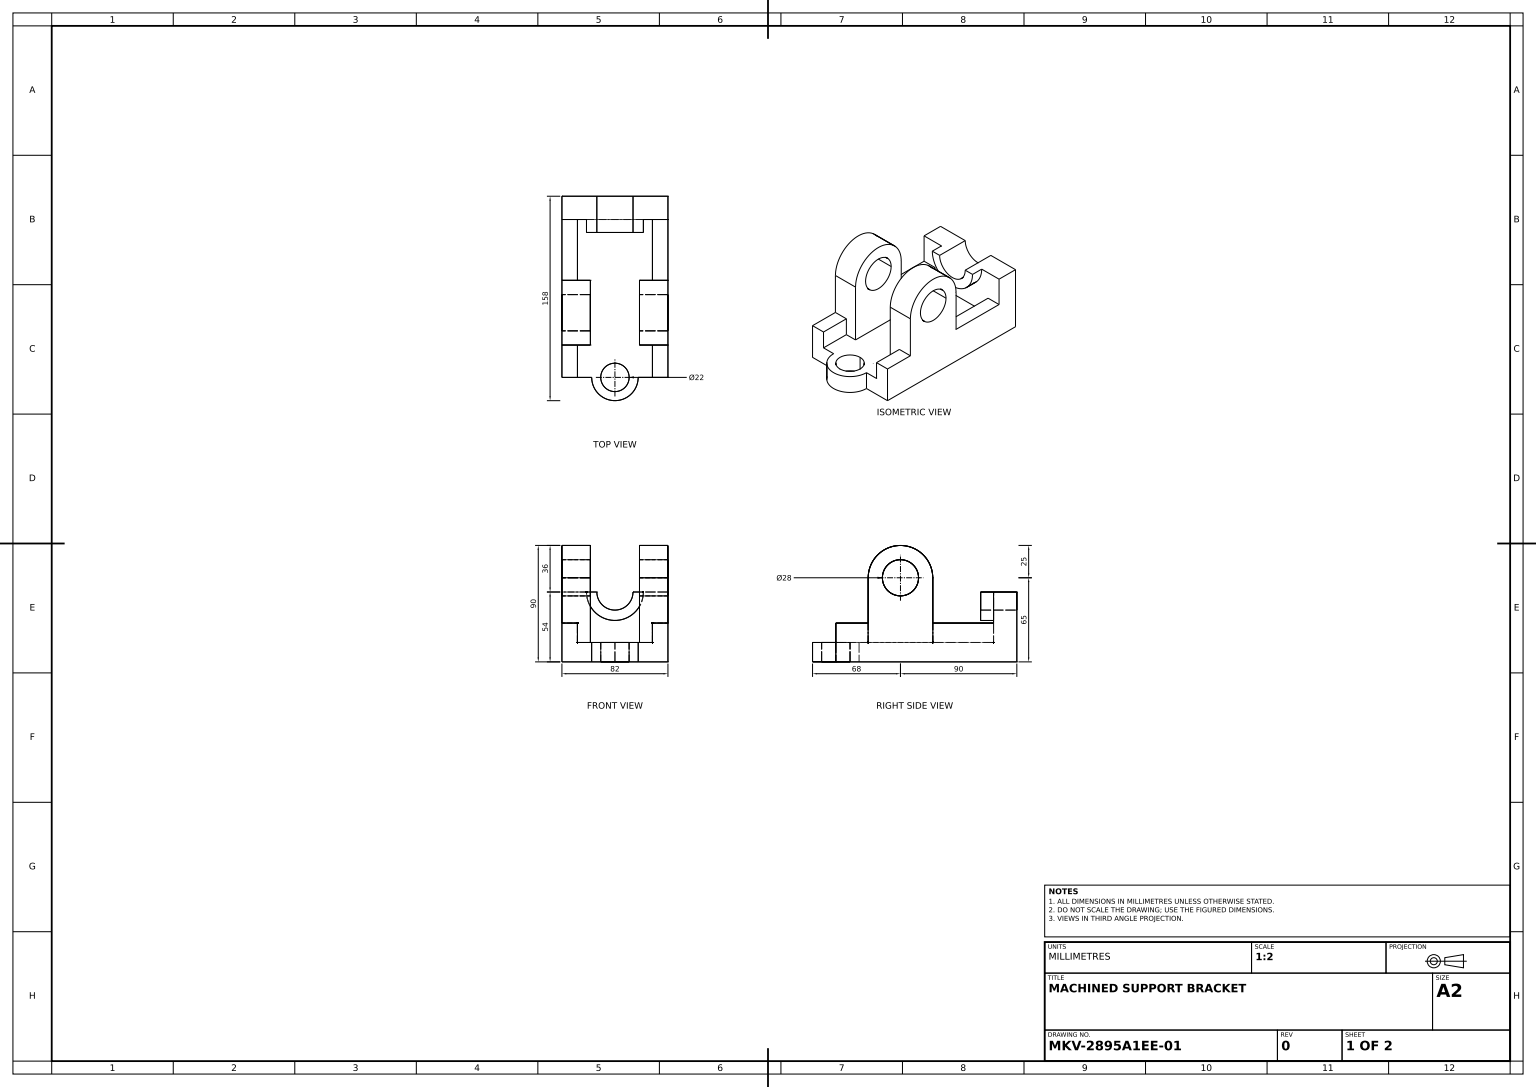
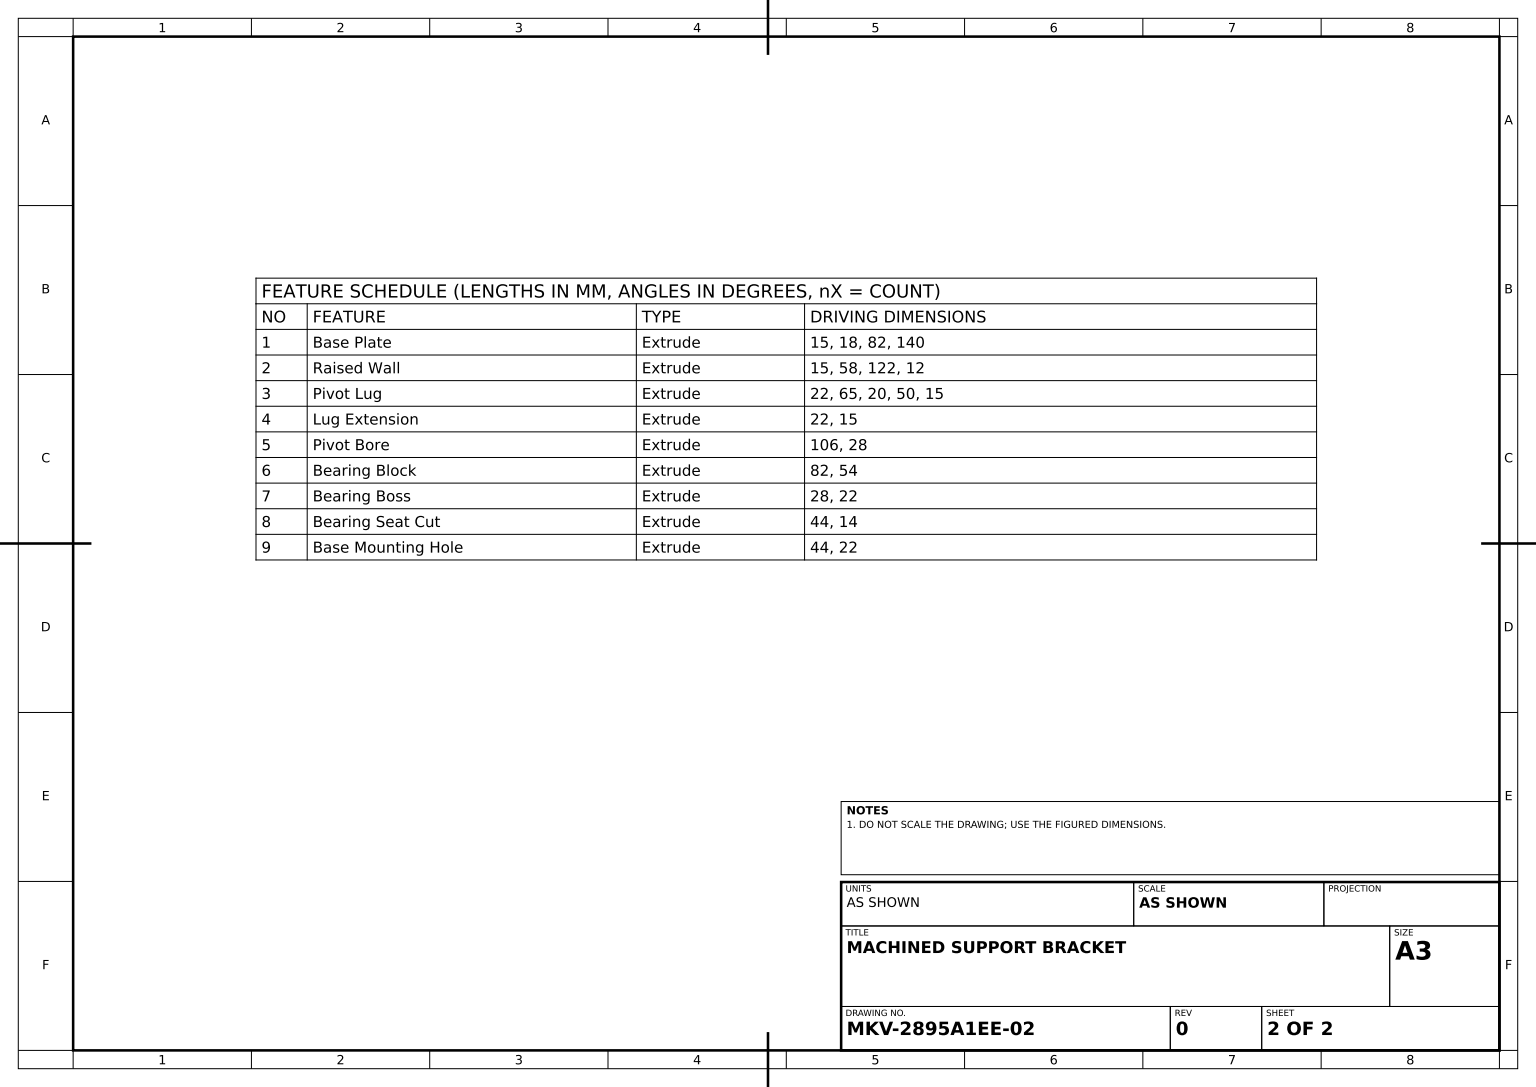
from build123d import *

# Parameters (mm, degrees)
BASE_PLATE_DEPTH            = 15
RAISED_WALL_DEPTH           = 15
PIVOT_LUG_DEPTH             = 22
LUG_START                   = -22
LUG_EXTENSION_DEPTH         = 22
PIVOT_BORE_SKETCH_R         = 14
PIVOT_BORE_DEPTH            = 106
BEARING_BLOCK_DEPTH         = 82
BEARING_BOSS_DEPTH          = 28
BEARING_SEAT_CUT_DEPTH      = 44
BASE_MOUNTING_HOLE_SKETCH_R = 11
BASE_MOUNTING_HOLE_DEPTH    = 44


with BuildPart() as part:
    # Base Plate Sketch → Base Plate (new body)
    with BuildSketch(Plane(origin=(0, 0, 0), x_dir=(1, 0, 0), z_dir=(0, 1, 0))):
        with BuildLine():
            Line((18, -70), (41, -70))
            Line((41, -70), (41, 0))
            Line((41, 0), (41, 70))
            Line((41, 70), (-41, 70))
            Line((-41, 70), (-41, -70))
            Line((-41, -70), (-18, -70))
            ThreePointArc((-18, -70), (0, -88), (18, -70))
        make_face()
    extrude(amount=BASE_PLATE_DEPTH)

    # Raised Wall Sketch → Raised Wall (add)
    with BuildSketch(Plane(origin=(0, 15, 0), x_dir=(1, 0, 0), z_dir=(0, 1, 0))):
        Polygon((41, -70), (29, -70), (29, 52), (-29, 52), (-29, -70), (-41, -70), (-41, 70), (41, 70), align=None)
    extrude(amount=RAISED_WALL_DEPTH)

    # Pivot Lug Sketch → Pivot Lug (add)
    with BuildSketch(Plane.ZY.offset(41)):
        with BuildLine():
            Line((45, 30), (45, 15))
            Line((45, 15), (-5, 15))
            Line((-5, 15), (-5, 30))
            Line((-5, 30), (-5, 65))
            ThreePointArc((-5, 65), (20, 90), (45, 65))
            Line((45, 65), (45, 30))
        make_face()
    extrude(amount=-PIVOT_LUG_DEPTH)

    # Lug Extension Sketch → Lug Extension (add)
    with BuildSketch(Plane(origin=(41, 0, 0), x_dir=(0, 0, -1), z_dir=(1, 0, 0)).offset(LUG_START)):
        with BuildLine():
            Line((5, 15), (-20, 15))
            Line((-20, 15), (-45, 15))
            Line((-45, 15), (-45, 65))
            ThreePointArc((-45, 65), (-20, 90), (5, 65))
            Line((5, 65), (5, 15))
        make_face()
    extrude(amount=LUG_EXTENSION_DEPTH)

    # Pivot Bore Sketch → Pivot Bore (cut)
    with BuildSketch(Plane.ZY.offset(41)):
        with Locations((20, 65)):
            Circle(PIVOT_BORE_SKETCH_R)
    extrude(amount=-PIVOT_BORE_DEPTH, mode=Mode.SUBTRACT)

    # Bearing Block Sketch → Bearing Block (add)
    with BuildSketch(Plane.ZY.offset(41)):
        Polygon((-70, 0), (-70, 54), (-52, 54), (-52, 30), (-52, 0), align=None)
    extrude(amount=-BEARING_BLOCK_DEPTH)

    # Bearing Boss Sketch → Bearing Boss (add)
    with BuildSketch(Plane(origin=(0, 0, -70), x_dir=(-1, 0, 0), z_dir=(0, 0, -1))):
        with BuildLine():
            Line((-22, 54), (22, 54))
            ThreePointArc((22, 54), (0, 32), (-22, 54))
        make_face()
    extrude(amount=-BEARING_BOSS_DEPTH)

    # Bearing Seat Sketch → Bearing Seat Cut (cut)
    with BuildSketch(Plane(origin=(0, 0, -70), x_dir=(-1, 0, 0), z_dir=(0, 0, -1))):
        with BuildLine():
            Line((-14, 54), (14, 54))
            ThreePointArc((14, 54), (0, 40), (-14, 54))
        make_face()
    extrude(amount=-BEARING_SEAT_CUT_DEPTH, mode=Mode.SUBTRACT)

    # Base Mounting Hole Sketch → Base Mounting Hole (cut)
    with BuildSketch(Plane(origin=(0, 15, 0), x_dir=(1, 0, 0), z_dir=(0, 1, 0))):
        with Locations(Location((0, -70, 0), (0, 0, 270))):
            Circle(BASE_MOUNTING_HOLE_SKETCH_R)
    extrude(amount=-BASE_MOUNTING_HOLE_DEPTH, mode=Mode.SUBTRACT)


solid = part.part
